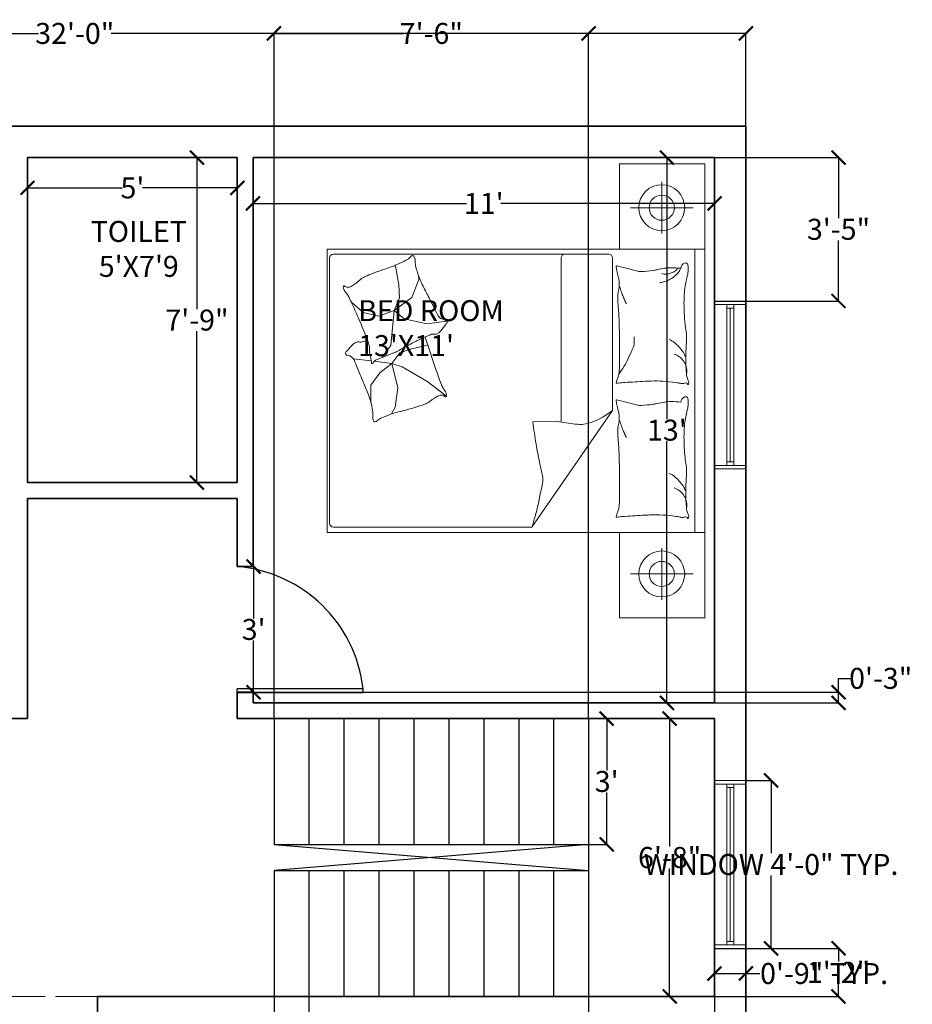
# Model space of a CAD drawing. Units: inches. Extents: x 43 to 543, y 36 to 629.
# Tile 5 of 5: x 261 to 516, y 348 to 629. Entities that reach past the tile are written whole.
import ezdxf

# ---------------------------------------------------------------- set-up
doc = ezdxf.new("R2010")
doc.units = ezdxf.units.IN
doc.header["$MEASUREMENT"] = 0
doc.linetypes.add('ACAD_ISO02W100', pattern=[15, 12, -3])
for name, color, linetype, lineweight in [('A-ANNO-DIMS', 2, 'Continuous', 18), ('A-AREA-IDEN', 7, 'Continuous', 25), ('A-DOOR', 3, 'Continuous', 25), ('A-FLOR-STRS', 7, 'Continuous', 25), ('A-FURN', 8, 'Continuous', 13), ('A-GLAZ', 4, 'Continuous', 18), ('A-WALL', 7, 'Continuous', 35), ('A-WALL-OVHD', 7, 'ACAD_ISO02W100', 18)]:
    doc.layers.add(name, color=color, linetype=linetype, lineweight=lineweight)
doc.styles.add('DIM_FONT', font='SIMPLEX.shx', dxfattribs={"width": 0.8})
doc.styles.get("Standard").update_dxf_attribs({"font": 'arial.ttf'})
doc.dimstyles.get("Standard").update_dxf_attribs({"dimtxt": 6, "dimasz": 4, "dimexe": 0.18, "dimexo": 0.0625, "dimgap": 0.09, "dimtad": 0, "dimtih": 1, "dimtoh": 1, "dimdec": 0, "dimzin": 0, "dimdsep": 46, "dimlunit": 4, "dimtxsty": 'Standard', "dimblk": 'ARCHTICK', "dimcen": 0.09, "dimadec": 0, "dimazin": 0, "dimtfac": 1, "dimtdec": 0, "dimtofl": 0, "dimtmove": 0, "dimatfit": 3, "dimldrblk": 'ARCHTICK', "dimfxl": 1, "dimtolj": 1, "dimtzin": 0, "dimarcsym": 1})

# ---------------------------------------------------------------- blocks, each defined once
blk = doc.blocks.new('XDCGFBHJNK')
for p, q in [((549.02, 46.3), (549.02, 41.8)), ((549.02, 46.3), (549.02, 10.3)), ((549.02, 46.3), (550.02, 46.3)), ((550.02, 10.3), (550.02, 46.3)), ((549.02, 10.3), (550.02, 10.3))]:
    blk.add_line(p, q)
blk.add_arc((545.53, 49.68), 39.64, 276.512, 355.1019)
blk = doc.blocks.new('TFHJBHN')
for p, q in [((347.02, 210.06), (338.02, 210.06)), ((347.02, 209.06), (338.02, 209.06)), ((341.52, 209.06), (341.52, 163.06)), ((343.52, 209.06), (343.52, 163.06)), ((343.52, 208.06), (341.52, 208.06)), ((342.52, 208.06), (342.52, 164.06)), ((341.52, 164.06), (343.52, 164.06)), ((338.02, 163.06), (347.02, 163.06)), ((338.02, 162.06), (347.02, 162.06))]:
    blk.add_line(p, q)
blk = doc.blocks.new('_ArchTick')
at = {"color": 0, "linetype": 'ByBlock', "const_width": 0.15}
blk.add_lwpolyline([(-0.5, -0.5), (0.5, 0.5)], dxfattribs=at)
blk = doc.blocks.new('*D4')
at = {"layer": 'A-ANNO-DIMS', "color": 0, "lineweight": -2, "transparency": 16777216}
for p, q in [((327.88, 589.95), (327.88, 576.71)), ((459.88, 589.95), (459.88, 576.71)), ((327.88, 576.89), (388.98, 576.89)), ((459.88, 576.89), (398.78, 576.89))]:
    blk.add_line(p, q, dxfattribs=at)
at = {"layer": 'Defpoints', "color": 0, "transparency": 16777216}
for p in [(327.88, 590.02), (459.88, 590.02), (459.88, 576.89)]:
    blk.add_point(p, dxfattribs=at)
at = {"layer": 'A-ANNO-DIMS', "color": 0, "lineweight": -2, "transparency": 16777216, "xscale": 4, "yscale": 4, "zscale": 4, "rotation": 180}
blk.add_blockref('_ArchTick', (327.88, 576.89), dxfattribs=at)
at = {"layer": 'A-ANNO-DIMS', "color": 0, "lineweight": -2, "transparency": 16777216, "xscale": 4, "yscale": 4, "zscale": 4}
blk.add_blockref('_ArchTick', (459.88, 576.89), dxfattribs=at)
at = {"layer": 'A-ANNO-DIMS', "color": 0, "transparency": 16777216, "insert": (393.88, 576.89), "char_height": 6, "attachment_point": 5}
blk.add_mtext("\\A1;11'", dxfattribs=at)
blk = doc.blocks.new('*D5')
at = {"layer": 'A-ANNO-DIMS', "color": 0, "lineweight": -2, "transparency": 16777216}
for p, q in [((459.82, 590.02), (446.09, 590.02)), ((446.27, 590.02), (446.27, 515.17)), ((446.27, 434.02), (446.27, 508.86)), ((459.82, 434.02), (446.09, 434.02))]:
    blk.add_line(p, q, dxfattribs=at)
at = {"layer": 'Defpoints', "color": 0, "transparency": 16777216}
for p in [(459.88, 590.02), (446.27, 434.02), (459.88, 434.02)]:
    blk.add_point(p, dxfattribs=at)
at = {"layer": 'A-ANNO-DIMS', "color": 0, "lineweight": -2, "transparency": 16777216, "xscale": 4, "yscale": 4, "zscale": 4}
for p, rotation in [((446.27, 590.02), 90), ((446.27, 434.02), 270)]:
    blk.add_blockref('_ArchTick', p, dxfattribs=dict(at, rotation=rotation))
at = {"layer": 'A-ANNO-DIMS', "color": 0, "transparency": 16777216, "insert": (446.27, 512.02), "char_height": 6, "attachment_point": 5}
blk.add_mtext("\\A1;13'", dxfattribs=at)
blk = doc.blocks.new('*D6')
at = {"layer": 'A-ANNO-DIMS', "color": 0, "lineweight": -2, "transparency": 16777216}
for p, q in [((263.38, 589.95), (263.38, 581.15)), ((323.38, 589.95), (323.38, 581.15)), ((263.38, 581.33), (290.53, 581.33)), ((323.38, 581.33), (296.23, 581.33))]:
    blk.add_line(p, q, dxfattribs=at)
at = {"layer": 'Defpoints', "color": 0, "transparency": 16777216}
for p in [(263.38, 590.02), (323.38, 590.02), (323.38, 581.33)]:
    blk.add_point(p, dxfattribs=at)
at = {"layer": 'A-ANNO-DIMS', "color": 0, "lineweight": -2, "transparency": 16777216, "xscale": 4, "yscale": 4, "zscale": 4, "rotation": 180}
blk.add_blockref('_ArchTick', (263.38, 581.33), dxfattribs=at)
at = {"layer": 'A-ANNO-DIMS', "color": 0, "lineweight": -2, "transparency": 16777216, "xscale": 4, "yscale": 4, "zscale": 4}
blk.add_blockref('_ArchTick', (323.38, 581.33), dxfattribs=at)
at = {"layer": 'A-ANNO-DIMS', "color": 0, "transparency": 16777216, "insert": (293.38, 581.33), "char_height": 6, "attachment_point": 5}
blk.add_mtext("\\A1;5'", dxfattribs=at)
blk = doc.blocks.new('*D7')
at = {"layer": 'A-ANNO-DIMS', "color": 0, "lineweight": -2, "transparency": 16777216}
for p, q in [((323.32, 590.02), (311.66, 590.02)), ((311.84, 590.02), (311.84, 546.67)), ((311.84, 497.02), (311.84, 540.36)), ((323.32, 497.02), (311.66, 497.02))]:
    blk.add_line(p, q, dxfattribs=at)
at = {"layer": 'Defpoints', "color": 0, "transparency": 16777216}
for p in [(323.38, 590.02), (311.84, 497.02), (323.38, 497.02)]:
    blk.add_point(p, dxfattribs=at)
at = {"layer": 'A-ANNO-DIMS', "color": 0, "lineweight": -2, "transparency": 16777216, "xscale": 4, "yscale": 4, "zscale": 4}
for p, rotation in [((311.84, 590.02), 90), ((311.84, 497.02), 270)]:
    blk.add_blockref('_ArchTick', p, dxfattribs=dict(at, rotation=rotation))
at = {"layer": 'A-ANNO-DIMS', "color": 0, "transparency": 16777216, "insert": (311.84, 543.52), "char_height": 6, "attachment_point": 5}
blk.add_mtext('\\A1;7\'-9"', dxfattribs=at)
blk = doc.blocks.new('*D16')
at = {"layer": 'A-ANNO-DIMS', "color": 0, "lineweight": -2, "transparency": 16777216}
for p, q in [((459.82, 429.52), (446.88, 429.52)), ((447.06, 429.52), (447.06, 392.92)), ((447.06, 350.02), (447.06, 386.61)), ((459.82, 350.02), (446.88, 350.02))]:
    blk.add_line(p, q, dxfattribs=at)
at = {"layer": 'Defpoints', "color": 0, "transparency": 16777216}
for p in [(459.88, 429.52), (447.06, 350.02), (459.88, 350.02)]:
    blk.add_point(p, dxfattribs=at)
at = {"layer": 'A-ANNO-DIMS', "color": 0, "lineweight": -2, "transparency": 16777216, "xscale": 4, "yscale": 4, "zscale": 4}
for p, rotation in [((447.06, 429.52), 90), ((447.06, 350.02), 270)]:
    blk.add_blockref('_ArchTick', p, dxfattribs=dict(at, rotation=rotation))
at = {"layer": 'A-ANNO-DIMS', "color": 0, "transparency": 16777216, "insert": (447.06, 389.77), "char_height": 6, "attachment_point": 5}
blk.add_mtext('\\A1;6\'-8"', dxfattribs=at)
blk = doc.blocks.new('*D17')
at = {"layer": 'A-ANNO-DIMS', "color": 0, "lineweight": -2, "transparency": 16777216}
for p, q in [((413.94, 429.52), (429.23, 429.52)), ((429.05, 429.52), (429.05, 414.67)), ((429.05, 393.52), (429.05, 408.36)), ((413.94, 393.52), (429.23, 393.52))]:
    blk.add_line(p, q, dxfattribs=at)
at = {"layer": 'Defpoints', "color": 0, "transparency": 16777216}
for p in [(413.88, 429.52), (413.88, 393.52), (429.05, 393.52)]:
    blk.add_point(p, dxfattribs=at)
at = {"layer": 'A-ANNO-DIMS', "color": 0, "lineweight": -2, "transparency": 16777216, "xscale": 4, "yscale": 4, "zscale": 4}
for p, rotation in [((429.05, 429.52), 90), ((429.05, 393.52), 270)]:
    blk.add_blockref('_ArchTick', p, dxfattribs=dict(at, rotation=rotation))
at = {"layer": 'A-ANNO-DIMS', "color": 0, "transparency": 16777216, "insert": (429.05, 411.52), "char_height": 6, "attachment_point": 5}
blk.add_mtext("\\A1;3'", dxfattribs=at)
blk = doc.blocks.new('*D18')
at = {"layer": 'A-ANNO-DIMS', "color": 0, "lineweight": -2, "transparency": 16777216}
for p, q in [((323.44, 473.02), (328.23, 473.02)), ((328.05, 473.02), (328.05, 458.17)), ((328.05, 437.02), (328.05, 451.86)), ((323.44, 437.02), (328.23, 437.02))]:
    blk.add_line(p, q, dxfattribs=at)
at = {"layer": 'Defpoints', "color": 0, "transparency": 16777216}
for p in [(323.38, 473.02), (323.38, 437.02), (328.05, 437.02)]:
    blk.add_point(p, dxfattribs=at)
at = {"layer": 'A-ANNO-DIMS', "color": 0, "lineweight": -2, "transparency": 16777216, "xscale": 4, "yscale": 4, "zscale": 4}
for p, rotation in [((328.05, 473.02), 90), ((328.05, 437.02), 270)]:
    blk.add_blockref('_ArchTick', p, dxfattribs=dict(at, rotation=rotation))
at = {"layer": 'A-ANNO-DIMS', "color": 0, "transparency": 16777216, "insert": (328.05, 455.02), "char_height": 6, "attachment_point": 5}
blk.add_mtext("\\A1;3'", dxfattribs=at)
blk = doc.blocks.new('BED-DOUBLE-WITH-NIGHTSTANDS')
for p, q in [((83.62, 105.4), (83.62, 129.79)), ((83.62, 129.79), (108, 129.79)), ((108, 129.79), (108, 105.4)), ((95.68, 109.93), (95.68, 124.65)), ((104.67, 117.29), (86.69, 117.29)), ((105.17, 105.4), (105.17, 24.4)), ((0.66, 102.92), (0.66, 27.01)), ((80.54, 104), (1.74, 104)), ((66.9, 102.92), (66.9, 55.97)), ((81.62, 59.31), (81.62, 102.92)), ((19.54, 100.52), (19.19, 100.7)), ((20.47, 95.22), (19.54, 100.52)), ((24.18, 91.6), (26.22, 96.71)), ((26.22, 96.71), (26.04, 98.01)), ((20.65, 91.51), (20.47, 95.22)), ((10.26, 87.33), (6.88, 90.22)), ((19.17, 87.89), (24.18, 91.6)), ((19.17, 87.89), (20.65, 91.51)), ((14.71, 86.21), (10.26, 87.33)), ((19.17, 87.89), (14.71, 86.21)), ((19.17, 87.89), (18.15, 77.85)), ((21.95, 85.47), (19.17, 87.89)), ((28.54, 84.08), (21.95, 85.47)), ((34.11, 84.82), (28.54, 84.08)), ((18.15, 77.85), (16.2, 75.16)), ((20.71, 75.8), (23.8, 76.86)), ((23.8, 76.86), (28.6, 77.93)), ((12.59, 73.43), (7.48, 74.07)), ((18.47, 72.7), (13.38, 73.34)), ((16.2, 75.16), (15.73, 74.51)), ((18.47, 72.7), (20.71, 75.8)), ((18.47, 72.7), (15.05, 70.03)), ((21.45, 71.74), (18.47, 72.7)), ((18.47, 72.7), (20.17, 65.76)), ((28.49, 67.68), (21.45, 71.74)), ((15.05, 70.03), (12.49, 66.51)), ((34.11, 63.41), (28.49, 67.68)), ((12.49, 66.51), (12.49, 61.49)), ((20.17, 65.76), (19.43, 60.21)), ((19.43, 60.21), (18.34, 58.27)), ((81.62, 59.31), (58.54, 25.93)), ((1.74, 25.93), (58.54, 25.93)), ((83.62, 24.4), (83.62, 0)), ((108, 0), (108, 24.4)), ((95.68, 19.86), (95.68, 5.14)), ((104.67, 12.5), (86.69, 12.5)), ((83.62, 0), (108, 0))]:
    blk.add_line(p, q)
blk.add_lwpolyline([(0, 105.4), (108, 105.4), (108, 24.4), (0, 24.4)], close=True)
blk.add_lwpolyline([(22.51, 102.26, 0.101392), (23.8, 103.26, -0.223768), (24.5, 103.58, -0.25558), (24.77, 103.43, -0.081563), (25.1, 102.61, -0.071805), (25.18, 101.69, 0.069985), (25.26, 100.74, 0.03546), (26.2, 97.59, 0.029432), (27.82, 93.98, 0.001554), (28.73, 92.24, -0.00152), (29.66, 90.47, -0.004735), (30.6, 88.63, 0.00382), (31.75, 86.35, 0.296001), (33.58, 85.3, -0.649774), (34.16, 84.19, -0.02319), (33.93, 83.92, 0.0288), (33.74, 83.71, 0.005727), (33.46, 83.33, -0.004358), (33.09, 82.83, -0.027528), (32.25, 81.85, -0.046214), (31.67, 81.34, -0.194121), (30.78, 81.12, 0.133719), (29.49, 80.96, 0.011505), (27.21, 79.95, 0.008882), (24.3, 78.53, 0.012426), (20.61, 76.53, -0.033612), (19.21, 75.84), (16.17, 74.6), (13.82, 73.64, 0.224341), (13.11, 72.86, -0.722772), (12.63, 72.85, -0.103513), (12.6, 73.05, 0.053465), (12.59, 73.44, 0.030109), (12.34, 74.68, -0.031436), (12.1, 75.88, -0.05324), (12.08, 76.69, 0.05518), (12.05, 77.48, 0.056271), (11.7, 78.85, 0.0108), (8.92, 85.64, 0.00456), (6.88, 90.22, 0.01125), (5.99, 92.05, 0.069394), (5.31, 93.02, -0.079756), (4.74, 93.88, -0.106399), (4.57, 94.66, -0.328642), (4.73, 94.89, -0.299547), (5.09, 94.79, 0.189917), (5.59, 94.53, 0.033518), (6.15, 94.51, 0.075627), (6.39, 94.55, 0.053489), (6.8, 94.74, 0.017838), (7.94, 95.49, 0.038394), (9.17, 96.51, -0.059529), (10, 97.14, -0.035943), (11.36, 97.82, -0.011245), (15.91, 99.56, -0.006203), (17.99, 100.27, 0.010783), (19.19, 100.7, 0.019485), (19.89, 100.99, 0.005062)], format="xyb", close=True)
for points in [[(101.15, 99.94, -0.263368), (102.17, 101.45, -0.494818), (103.18, 100.96, -0.049225), (103.27, 100, -0.036831), (103.18, 98.73, -0.031893), (102.74, 96.68, 0.035782), (102.36, 94.84, 0.032941), (102.04, 90, 0.026564), (102.36, 84, 0.017905), (102.65, 81.97, -0.033397), (102.77, 80.88, -0.03204), (102.73, 78.88, 0.018442), (102.57, 75.4, 0.010837), (102.61, 71.91, 0.014624), (102.77, 69.32, 0.111249), (103.17, 68.1, -0.153708), (103.38, 67.19, -0.076444), (103.29, 66.79, -0.215512), (103.18, 66.68, -0.585858), (103.02, 66.83, 0.363489), (102.88, 67.09, 0.191716), (102.25, 67.09, -0.129675), (101.36, 66.99, -0.01735), (100.45, 67.15, 0.019326), (99.63, 67.29, 0.018818), (95.94, 67.65, 0.021828), (92.74, 67.7, 0.006204), (90.91, 67.62, 0.001963), (85.14, 67.29, 0.028341), (83.19, 67.06, -0.117014), (82.71, 67.09, -0.36606), (82.66, 67.17, -0.03973), (82.81, 67.9, -0.048309), (83.11, 68.64, 0.062981), (83.32, 69.22, 0.04058), (83.5, 70.48, 0.014345), (83.62, 74.08, 0.005484), (83.58, 80.86, 0.007153), (83.42, 86.05, 0.008762), (83.27, 88.35, -0.008153), (83.12, 90.82, -0.06251), (83.35, 93.9, 0.078669), (83.46, 96.36, 0.047825), (83.21, 97.57, -0.034494), (82.81, 99.23, -0.023571), (82.65, 100.6, -0.510228), (82.71, 100.65), (84.33, 100.25), (88.79, 99.13, 0.073041), (89.85, 99.03, 0.023305), (93.15, 99.33, 0.018299), (94.38, 99.55, -0.01097), (96.43, 99.95, -0.042281), (98.29, 100.11, -0.027201), (101.17, 99.95)], [(101.15, 99.95, -0.077379), (99.79, 98.07, -0.077379), (97.91, 96.7, -0.047525), (96.58, 96.16, -0.047525), (95.17, 95.89)], [(100.29, 100.03, -0.05369), (99.59, 99.27, -0.070312), (98.92, 98.83, -0.015448), (98.46, 98.63, -0.013244), (97.91, 98.42, -0.082127), (96.93, 98.26, -0.064164), (95.68, 98.42)], [(83.5, 95.06, 0.009729), (83.99, 93.59, 0.009729), (84.53, 92.13, 0.007971), (85.02, 90.96, 0.007971), (85.55, 89.8)], [(28.06, 80.34, 0.025626), (28.21, 79.72, 0.0108), (30.46, 72.73, 0.00456), (32.14, 68.01, 0.01125), (32.88, 66.11, 0.069394), (33.49, 65.1, -0.079756), (33.99, 64.2, -0.106399), (34.11, 63.41, -0.328642), (33.92, 63.19, -0.299547), (33.57, 63.32, 0.189917), (33.1, 63.62, 0.033518), (32.54, 63.68, 0.075627), (32.29, 63.65, 0.053489), (31.87, 63.49, 0.017838), (30.68, 62.84, 0.038394), (29.37, 61.91, -0.059529), (28.5, 61.35, -0.035943), (27.09, 60.78, -0.011245), (22.42, 59.39, -0.006203), (20.29, 58.84, 0.010783), (19.06, 58.51, 0.019485), (18.34, 58.27, 0.005062), (15.63, 57.21, 0.101392), (14.27, 56.3, -0.223768), (13.54, 56.04, -0.25558), (13.29, 56.21, -0.081563), (13.02, 57.06, -0.071805), (13.01, 57.98, 0.069985), (13.01, 58.93, 0.03546), (12.31, 62.14, 0.029432), (10.97, 65.87, 0.001554), (10.2, 67.67, -0.00152), (9.41, 69.51, -0.004735), (8.61, 71.41, 0.00382), (7.64, 73.78, 0.296001), (5.89, 74.96, -0.649774), (5.41, 76.12, -0.02319), (5.66, 76.36, 0.0288), (5.85, 76.56, 0.005727), (6.17, 76.91, -0.004358), (6.58, 77.38, -0.027528), (7.49, 78.3, -0.046214), (8.1, 78.76, -0.194121), (9, 78.91, 0.133719), (10.3, 78.98, 0.005779), (11.49, 79.38, 0.008882)], [(83.42, 69.72, 0.016108), (84.84, 71.83, 0.024599), (85.65, 73.27, 0.009477), (86.91, 75.92, 0.015937), (87.57, 77.53, 0.072521), (87.77, 78.41, 0.033339), (87.78, 80.37)], [(102.57, 74.35, 0.027842), (101.99, 75.64, 0.048685), (101.56, 76.32, 0.023666), (100.24, 77.82, 0.031223), (99.13, 78.85, 0.046801), (98.71, 79.13, 0.023191), (97.81, 79.56)], [(102.88, 69.93, 0.088153), (102.68, 71.79, 0.088153), (101.86, 73.48, 0.077547), (100.7, 74.65, 0.077547), (99.23, 75.4)], [(101.15, 61.64, -0.263368), (102.17, 63.15, -0.494818), (103.18, 62.66, -0.049225), (103.27, 61.7, -0.036831), (103.18, 60.43, -0.031893), (102.74, 58.38, 0.035782), (102.36, 56.55, 0.032941), (102.04, 51.7, 0.026564), (102.36, 45.7, 0.017905), (102.65, 43.67, -0.033397), (102.77, 42.58, -0.03204), (102.73, 40.58, 0.018442), (102.57, 37.1, 0.010837), (102.61, 33.61, 0.014624), (102.77, 31.02, 0.111249), (103.17, 29.8, -0.153708), (103.38, 28.89, -0.076444), (103.29, 28.49, -0.215512), (103.18, 28.38, -0.585858), (103.02, 28.53, 0.363489), (102.88, 28.79, 0.191716), (102.25, 28.79, -0.129675), (101.36, 28.69, -0.01735), (100.45, 28.85, 0.019326), (99.63, 28.99, 0.018818), (95.94, 29.35, 0.021828), (92.74, 29.4, 0.006204), (90.91, 29.32, 0.001963), (85.14, 28.99, 0.028341), (83.19, 28.76, -0.117014), (82.71, 28.79, -0.36606), (82.66, 28.87, -0.03973), (82.81, 29.6, -0.048309), (83.11, 30.34, 0.062981), (83.32, 30.92, 0.04058), (83.5, 32.18, 0.014345), (83.62, 35.79, 0.005484), (83.58, 42.56, 0.007153), (83.42, 47.75, 0.008762), (83.27, 50.05, -0.008153), (83.12, 52.52, -0.06251), (83.35, 55.6, 0.078669), (83.46, 58.06, 0.047825), (83.21, 59.27, -0.034494), (82.81, 60.93, -0.023571), (82.65, 62.3, -0.510228), (82.71, 62.35), (84.33, 61.95), (88.79, 60.83, 0.073041), (89.85, 60.73, 0.023305), (93.15, 61.04, 0.018299), (94.38, 61.26, -0.01097), (96.43, 61.65, -0.042281), (98.29, 61.81, -0.027201), (101.17, 61.65)], [(81.62, 59.31, -0.085272), (75.67, 55.89, -0.124044), (70.95, 55.39), (65.79, 56.13), (58.77, 56.03)], [(83.5, 56.76, 0.009729), (83.99, 55.29, 0.009729), (84.53, 53.84, 0.007971), (85.02, 52.66, 0.007971), (85.55, 51.5)], [(58.77, 56.03, 0.007867), (59.73, 49.68, 0.009508), (60.7, 44.46, 0.006616), (61.48, 40.95, -0.023828), (61.66, 39.97, -0.080713), (61.63, 38.96, -0.009591), (59.91, 30.72, -0.013133), (59.44, 28.91, -0.007859), (58.54, 25.93)], [(102.57, 36.06, 0.027842), (101.99, 37.34, 0.048685), (101.56, 38.02, 0.023666), (100.24, 39.52, 0.031223), (99.13, 40.55, 0.046801), (98.71, 40.83, 0.023191), (97.81, 41.26)], [(102.88, 31.63, 0.088153), (102.68, 33.49, 0.088153), (101.86, 35.18, 0.077547), (100.7, 36.35, 0.077547), (99.23, 37.1)]]:
    blk.add_lwpolyline(points, format="xyb")
for centre, radius in [((95.68, 117.29), 6.58), ((95.68, 117.29), 3.6), ((95.68, 12.5), 6.58), ((95.68, 12.5), 3.6)]:
    blk.add_circle(centre, radius)
for centre, start, end in [((1.74, 102.92), 90, 180), ((67.98, 102.92), 90, 180), ((80.54, 102.92), 0, 90), ((1.74, 27.01), 180, 270)]:
    blk.add_arc(centre, 1.08, start, end)
at = {"style": 'DIM_FONT', "width": 0.8, "flags": 9}
for tag in ['YSIZE', 'XSIZE']:
    blk.add_attdef(tag, (108, 105.4), '', height=0.027, rotation=270, dxfattribs=at)
blk = doc.blocks.new('*D35')
at = {"layer": 'A-ANNO-DIMS', "color": 0, "lineweight": -2, "transparency": 16777216}
for p, q in [((468.94, 411.78), (476.26, 411.78)), ((476.08, 411.78), (476.08, 390.98)), ((476.08, 363.78), (476.08, 384.59)), ((468.94, 363.78), (476.26, 363.78))]:
    blk.add_line(p, q, dxfattribs=at)
at = {"layer": 'Defpoints', "color": 0, "transparency": 16777216}
for p in [(468.88, 411.78), (476.08, 411.78), (468.88, 363.78)]:
    blk.add_point(p, dxfattribs=at)
at = {"layer": 'A-ANNO-DIMS', "color": 0, "lineweight": -2, "transparency": 16777216, "xscale": 4, "yscale": 4, "zscale": 4}
for p, rotation in [((476.08, 411.78), 90), ((476.08, 363.78), 270)]:
    blk.add_blockref('_ArchTick', p, dxfattribs=dict(at, rotation=rotation))
at = {"layer": 'A-ANNO-DIMS', "color": 0, "transparency": 16777216, "insert": (476.08, 387.78), "char_height": 6, "attachment_point": 5}
blk.add_mtext('\\A1;WINDOW 4\'-0" TYP.', dxfattribs=at)
blk = doc.blocks.new('*D36')
at = {"layer": 'A-ANNO-DIMS', "color": 0, "lineweight": -2, "transparency": 16777216}
for p, q in [((459.88, 363.72), (459.88, 356.4)), ((468.88, 363.72), (468.88, 356.4)), ((459.88, 356.58), (468.88, 356.58)), ((468.88, 356.58), (472.88, 356.58))]:
    blk.add_line(p, q, dxfattribs=at)
at = {"layer": 'Defpoints', "color": 0, "transparency": 16777216}
for p in [(459.88, 363.78), (468.88, 363.78), (468.88, 356.58)]:
    blk.add_point(p, dxfattribs=at)
at = {"layer": 'A-ANNO-DIMS', "color": 0, "lineweight": -2, "transparency": 16777216, "xscale": 4, "yscale": 4, "zscale": 4, "rotation": 180}
blk.add_blockref('_ArchTick', (459.88, 356.58), dxfattribs=at)
at = {"layer": 'A-ANNO-DIMS', "color": 0, "lineweight": -2, "transparency": 16777216, "xscale": 4, "yscale": 4, "zscale": 4}
blk.add_blockref('_ArchTick', (468.88, 356.58), dxfattribs=at)
at = {"layer": 'A-ANNO-DIMS', "color": 0, "transparency": 16777216, "insert": (491.25, 356.58), "char_height": 6, "attachment_point": 5}
blk.add_mtext('\\A1;0\'-9" TYP.', dxfattribs=at)
blk = doc.blocks.new('*D37')
at = {"layer": 'A-ANNO-DIMS', "color": 0, "lineweight": -2, "transparency": 16777216}
for p, q in [((84.88, 599.08), (84.88, 625.7)), ((84.88, 625.52), (266.48, 625.52)), ((468.88, 625.52), (287.27, 625.52)), ((468.88, 599.08), (468.88, 625.7))]:
    blk.add_line(p, q, dxfattribs=at)
at = {"layer": 'Defpoints', "color": 0, "transparency": 16777216}
for p in [(468.88, 625.52), (84.88, 599.02), (468.88, 599.02)]:
    blk.add_point(p, dxfattribs=at)
at = {"layer": 'A-ANNO-DIMS', "color": 0, "lineweight": -2, "transparency": 16777216, "xscale": 4, "yscale": 4, "zscale": 4, "rotation": 180}
blk.add_blockref('_ArchTick', (84.88, 625.52), dxfattribs=at)
at = {"layer": 'A-ANNO-DIMS', "color": 0, "lineweight": -2, "transparency": 16777216, "xscale": 4, "yscale": 4, "zscale": 4}
blk.add_blockref('_ArchTick', (468.88, 625.52), dxfattribs=at)
at = {"layer": 'A-ANNO-DIMS', "color": 0, "transparency": 16777216, "insert": (276.88, 625.52), "char_height": 6, "attachment_point": 5}
blk.add_mtext('\\A1;32\'-0"', dxfattribs=at)
blk = doc.blocks.new('*D39')
at = {"layer": 'A-ANNO-DIMS', "color": 0, "lineweight": -2, "transparency": 16777216}
for p, q in [((459.94, 590.02), (495.56, 590.02)), ((495.38, 590.02), (495.38, 572.64)), ((495.38, 548.96), (495.38, 566.33)), ((459.94, 548.96), (495.56, 548.96))]:
    blk.add_line(p, q, dxfattribs=at)
at = {"layer": 'Defpoints', "color": 0, "transparency": 16777216}
for p in [(459.88, 590.02), (459.88, 548.96), (495.38, 548.96)]:
    blk.add_point(p, dxfattribs=at)
at = {"layer": 'A-ANNO-DIMS', "color": 0, "lineweight": -2, "transparency": 16777216, "xscale": 4, "yscale": 4, "zscale": 4}
for p, rotation in [((495.38, 590.02), 90), ((495.38, 548.96), 270)]:
    blk.add_blockref('_ArchTick', p, dxfattribs=dict(at, rotation=rotation))
at = {"layer": 'A-ANNO-DIMS', "color": 0, "transparency": 16777216, "insert": (495.38, 569.49), "char_height": 6, "attachment_point": 5}
blk.add_mtext('\\A1;3\'-5"', dxfattribs=at)
blk = doc.blocks.new('*D40')
at = {"layer": 'A-ANNO-DIMS', "color": 0, "lineweight": -2, "transparency": 16777216}
for p, q in [((459.94, 363.78), (495.56, 363.78)), ((495.38, 363.78), (495.38, 360)), ((495.38, 350.02), (495.38, 353.8)), ((459.94, 350.02), (495.56, 350.02))]:
    blk.add_line(p, q, dxfattribs=at)
at = {"layer": 'Defpoints', "color": 0, "transparency": 16777216}
for p in [(459.88, 363.78), (495.38, 363.78), (459.88, 350.02)]:
    blk.add_point(p, dxfattribs=at)
at = {"layer": 'A-ANNO-DIMS', "color": 0, "lineweight": -2, "transparency": 16777216, "xscale": 4, "yscale": 4, "zscale": 4}
for p, rotation in [((495.38, 363.78), 90), ((495.38, 350.02), 270)]:
    blk.add_blockref('_ArchTick', p, dxfattribs=dict(at, rotation=rotation))
at = {"layer": 'A-ANNO-DIMS', "color": 0, "transparency": 16777216, "insert": (495.38, 356.9), "char_height": 6, "attachment_point": 5}
blk.add_mtext('\\A1;1\'-2"', dxfattribs=at)
blk = doc.blocks.new('*D46')
at = {"layer": 'A-ANNO-DIMS', "color": 0, "lineweight": -2, "transparency": 16777216}
for p, q in [((333.88, 429.58), (333.88, 625.7)), ((333.88, 625.52), (370.84, 625.52)), ((423.88, 625.52), (386.92, 625.52)), ((423.88, 429.58), (423.88, 625.7))]:
    blk.add_line(p, q, dxfattribs=at)
at = {"layer": 'Defpoints', "color": 0, "transparency": 16777216}
for p in [(423.88, 625.52), (333.88, 429.52), (423.88, 429.52)]:
    blk.add_point(p, dxfattribs=at)
at = {"layer": 'A-ANNO-DIMS', "color": 0, "lineweight": -2, "transparency": 16777216, "xscale": 4, "yscale": 4, "zscale": 4, "rotation": 180}
blk.add_blockref('_ArchTick', (333.88, 625.52), dxfattribs=at)
at = {"layer": 'A-ANNO-DIMS', "color": 0, "lineweight": -2, "transparency": 16777216, "xscale": 4, "yscale": 4, "zscale": 4}
blk.add_blockref('_ArchTick', (423.88, 625.52), dxfattribs=at)
at = {"layer": 'A-ANNO-DIMS', "color": 0, "transparency": 16777216, "insert": (378.88, 625.52), "char_height": 6, "attachment_point": 5}
blk.add_mtext('\\A1;7\'-6"', dxfattribs=at)
blk = doc.blocks.new('*D47')
at = {"layer": 'A-ANNO-DIMS', "color": 0, "lineweight": -2, "transparency": 16777216}
for p, q in [((423.88, 349.95), (423.88, 44.34)), ((459.88, 349.95), (459.88, 44.34)), ((423.88, 44.52), (433.81, 44.52)), ((459.88, 44.52), (449.94, 44.52))]:
    blk.add_line(p, q, dxfattribs=at)
at = {"layer": 'Defpoints', "color": 0, "transparency": 16777216}
for p in [(423.88, 350.02), (459.88, 350.02), (459.88, 44.52)]:
    blk.add_point(p, dxfattribs=at)
at = {"layer": 'A-ANNO-DIMS', "color": 0, "lineweight": -2, "transparency": 16777216, "xscale": 4, "yscale": 4, "zscale": 4, "rotation": 180}
blk.add_blockref('_ArchTick', (423.88, 44.52), dxfattribs=at)
at = {"layer": 'A-ANNO-DIMS', "color": 0, "lineweight": -2, "transparency": 16777216, "xscale": 4, "yscale": 4, "zscale": 4}
blk.add_blockref('_ArchTick', (459.88, 44.52), dxfattribs=at)
at = {"layer": 'A-ANNO-DIMS', "color": 0, "transparency": 16777216, "insert": (441.88, 44.52), "char_height": 6, "attachment_point": 5}
blk.add_mtext('\\A1;3\'-0"', dxfattribs=at)
blk = doc.blocks.new('*D48')
at = {"layer": 'A-ANNO-DIMS', "color": 0, "lineweight": -2, "transparency": 16777216}
for p, q in [((333.88, 349.95), (333.88, 44.34)), ((343.88, 349.95), (343.88, 44.34)), ((333.88, 44.52), (343.88, 44.52)), ((343.88, 44.52), (347.88, 44.52))]:
    blk.add_line(p, q, dxfattribs=at)
at = {"layer": 'Defpoints', "color": 0, "transparency": 16777216}
for p in [(333.88, 350.02), (343.88, 350.02), (343.88, 44.52)]:
    blk.add_point(p, dxfattribs=at)
at = {"layer": 'A-ANNO-DIMS', "color": 0, "lineweight": -2, "transparency": 16777216, "xscale": 4, "yscale": 4, "zscale": 4, "rotation": 180}
blk.add_blockref('_ArchTick', (333.88, 44.52), dxfattribs=at)
at = {"layer": 'A-ANNO-DIMS', "color": 0, "lineweight": -2, "transparency": 16777216, "xscale": 4, "yscale": 4, "zscale": 4}
blk.add_blockref('_ArchTick', (343.88, 44.52), dxfattribs=at)
at = {"layer": 'A-ANNO-DIMS', "color": 0, "transparency": 16777216, "insert": (358.27, 44.52), "char_height": 6, "attachment_point": 5}
blk.add_mtext('\\A1;0\'-10"', dxfattribs=at)
blk = doc.blocks.new('*D63')
at = {"layer": 'A-ANNO-DIMS', "color": 0, "lineweight": -2, "transparency": 16777216}
for p, q in [((495.38, 437.02), (495.38, 441.02)), ((495.38, 441.02), (499.38, 441.02)), ((327.94, 437.02), (495.56, 437.02)), ((495.38, 434.02), (495.38, 437.02)), ((327.94, 434.02), (495.56, 434.02))]:
    blk.add_line(p, q, dxfattribs=at)
at = {"layer": 'Defpoints', "color": 0, "transparency": 16777216}
for p in [(327.88, 437.02), (495.38, 437.02), (327.88, 434.02)]:
    blk.add_point(p, dxfattribs=at)
at = {"layer": 'A-ANNO-DIMS', "color": 0, "lineweight": -2, "transparency": 16777216, "xscale": 4, "yscale": 4, "zscale": 4}
for p, rotation in [((495.38, 437.02), 90), ((495.38, 434.02), 270)]:
    blk.add_blockref('_ArchTick', p, dxfattribs=dict(at, rotation=rotation))
at = {"layer": 'A-ANNO-DIMS', "color": 0, "transparency": 16777216, "insert": (507.44, 441.02), "char_height": 6, "attachment_point": 5}
blk.add_mtext('\\A1;0\'-3"', dxfattribs=at)

msp = doc.modelspace()

# ---------------------------------------------------------------- linework, layer by layer
at = {"layer": 'A-FLOR-STRS'}
for p, q in [((333.88, 429.52), (333.88, 393.52)), ((343.88, 429.52), (343.88, 393.52)), ((353.88, 429.52), (353.88, 393.52)), ((363.88, 429.52), (363.88, 393.52)), ((373.88, 429.52), (373.88, 393.52)), ((383.88, 429.52), (383.88, 393.52)), ((393.88, 429.52), (393.88, 393.52)), ((403.88, 429.52), (403.88, 393.52)), ((413.88, 429.52), (413.88, 393.52)), ((423.88, 429.52), (423.88, 350.02)), ((333.88, 393.52), (423.88, 393.52)), ((423.88, 393.52), (333.88, 386.02)), ((333.88, 393.52), (423.88, 386.02)), ((333.88, 386.02), (423.88, 386.02)), ((333.88, 386.02), (333.88, 350.02)), ((343.88, 386.02), (343.88, 350.02)), ((353.88, 386.02), (353.88, 350.02)), ((363.88, 386.02), (363.88, 350.02)), ((373.88, 386.02), (373.88, 350.02)), ((383.88, 386.02), (383.88, 350.02)), ((393.88, 386.02), (393.88, 350.02)), ((403.88, 386.02), (403.88, 350.02)), ((413.88, 386.02), (413.88, 350.02))]:
    msp.add_line(p, q, dxfattribs=at)
at = {"layer": 'A-WALL'}
for p, q in [((84.88, 599.02), (468.88, 599.02)), ((468.88, 599.02), (468.88, 71.02)), ((263.38, 590.02), (263.38, 497.02)), ((263.38, 590.02), (323.38, 590.02)), ((323.38, 590.02), (323.38, 497.02)), ((327.88, 590.02), (327.88, 473.02)), ((327.88, 590.02), (459.88, 590.02)), ((459.88, 590.02), (459.88, 434.02)), ((323.38, 497.02), (263.38, 497.02)), ((323.38, 492.52), (263.38, 492.52)), ((263.38, 492.52), (263.38, 429.52)), ((323.38, 492.52), (323.38, 473.02)), ((323.38, 473.02), (327.88, 473.02)), ((323.38, 437.02), (327.88, 437.02)), ((323.38, 437.02), (323.38, 429.52)), ((327.88, 437.02), (327.88, 434.02)), ((327.88, 434.02), (459.88, 434.02)), ((258.88, 429.52), (263.38, 429.52)), ((323.38, 429.52), (459.88, 429.52)), ((459.88, 429.52), (459.88, 350.02)), ((283.38, 350.02), (283.38, 345.52)), ((283.38, 350.02), (459.88, 350.02))]:
    msp.add_line(p, q, dxfattribs=at)
at = {"layer": 'A-WALL-OVHD'}
msp.add_line((283.38, 350.02), (223.38, 350.02), dxfattribs=at)

# ---------------------------------------------------------------- block references
at = {"layer": 'A-DOOR', "rotation": 90}
msp.add_blockref('XDCGFBHJNK', (369.67, -112.01), dxfattribs=at)
at = {"layer": 'A-FURN'}
msp.add_blockref('BED-DOUBLE-WITH-NIGHTSTANDS', (349.13, 458.38), dxfattribs=at)
at = {"layer": 'A-GLAZ'}
for p in [(121.86, 338.9), (121.86, 201.72)]:
    msp.add_blockref('TFHJBHN', p, dxfattribs=at)

# ---------------------------------------------------------------- texts
at = {"layer": 'A-AREA-IDEN', "char_height": 6, "attachment_point": 1}
for s, width, insert in [("\\pxqc;TOILET\\P5'X7'9", 52.429, (268.98, 571.88)), ("BED ROOM\\P13'X11' ", 90.4757, (357.95, 549.21))]:
    msp.add_mtext_dynamic_manual_height_columns(s, width=width, gutter_width=30, heights=[0], dxfattribs=dict(at, insert=insert))

# ---------------------------------------------------------------- dimensions: what is measured, and where the dimension line sits
at = {"layer": 'A-ANNO-DIMS'}
for base, p1, p2, override, picture, middle in [((468.88, 625.52), (84.88, 599.02), (468.88, 599.02), {"dimdec": 1, "dimlfac": 1, "dimrnd": 0, "dimzin": 1, "dimdsep": 46, "dimlunit": 4, "dimfrac": 2}, '*D37', (276.88, 625.52)), ((423.88, 625.52), (333.88, 429.52), (423.88, 429.52), {"dimdec": 1, "dimlfac": 1, "dimrnd": 0, "dimzin": 1, "dimdsep": 46, "dimlunit": 4, "dimfrac": 2}, '*D46', (378.88, 625.52)), ((323.38, 581.33), (263.38, 590.02), (323.38, 590.02), {"dimclrd": 0, "dimclre": 0, "dimclrt": 0}, '*D6', (293.38, 581.33)), ((459.88, 576.89), (327.88, 590.02), (459.88, 590.02), {"dimclrd": 0, "dimclre": 0, "dimclrt": 0}, '*D4', (393.88, 576.89)), ((343.88, 44.52), (333.88, 350.02), (343.88, 350.02), {"dimdec": 1, "dimlfac": 1, "dimrnd": 0, "dimzin": 1, "dimdsep": 46, "dimlunit": 4, "dimfrac": 2}, '*D48', (358.27, 44.52)), ((459.88, 44.52), (423.88, 350.02), (459.88, 350.02), {"dimdec": 1, "dimlfac": 1, "dimrnd": 0, "dimzin": 1, "dimdsep": 46, "dimlunit": 4, "dimfrac": 2}, '*D47', (441.88, 44.52))]:
    dim = msp.add_linear_dim(base=base, p1=p1, p2=p2, dimstyle='Standard', override=override, dxfattribs=at)
    dim.commit()
    dim.dimension.update_dxf_attribs({"geometry": picture, "text_midpoint": middle})
for base, p1, p2, override, picture, middle in [((311.84, 497.02), (323.38, 590.02), (323.38, 497.02), {"dimclrd": 0, "dimclre": 0, "dimclrt": 0}, '*D7', (311.84, 543.52)), ((446.27, 434.02), (459.88, 590.02), (459.88, 434.02), {"dimclrd": 0, "dimclre": 0, "dimclrt": 0}, '*D5', (446.27, 512.02)), ((495.38, 548.96), (459.88, 590.02), (459.88, 548.96), {"dimdec": 1, "dimlfac": 1, "dimrnd": 0, "dimzin": 1, "dimdsep": 46, "dimlunit": 4, "dimfrac": 2}, '*D39', (495.38, 569.49)), ((328.05, 437.02), (323.38, 473.02), (323.38, 437.02), {"dimclrd": 0, "dimclre": 0, "dimclrt": 0}, '*D18', (328.05, 455.02)), ((495.38, 437.02), (327.88, 434.02), (327.88, 437.02), {"dimdec": 1, "dimlfac": 1, "dimrnd": 0, "dimzin": 1, "dimdsep": 46, "dimlunit": 4, "dimfrac": 2}, '*D63', (507.44, 441.02)), ((429.05, 393.52), (413.88, 429.52), (413.88, 393.52), {"dimclrd": 0, "dimclre": 0, "dimclrt": 0}, '*D17', (429.05, 411.52)), ((447.06164371, 350.01657912), (459.877649, 429.51657912), (459.877649, 350.01657912), {"dimclrd": 0, "dimclre": 0, "dimclrt": 0}, '*D16', (447.06164371, 389.76657912)), ((495.38, 363.78), (459.88, 350.02), (459.88, 363.78), {"dimdec": 1, "dimlfac": 1, "dimrnd": 0, "dimzin": 1, "dimdsep": 46, "dimlunit": 4, "dimfrac": 2}, '*D40', (495.38, 356.9))]:
    dim = msp.add_linear_dim(base=base, p1=p1, p2=p2, angle=90, dimstyle='Standard', override=override, dxfattribs=at)
    dim.commit()
    dim.dimension.update_dxf_attribs({"geometry": picture, "text_midpoint": middle})
dim = msp.add_linear_dim(base=(476.08, 411.78), p1=(468.88, 363.78), p2=(468.88, 411.78), angle=90, text='WINDOW <> TYP.', dimstyle='Standard', override={"dimdec": 1, "dimlfac": 1, "dimrnd": 0, "dimzin": 1, "dimdsep": 46, "dimlunit": 4, "dimfrac": 2}, dxfattribs=at)
dim.commit()
dim.dimension.update_dxf_attribs({"geometry": '*D35', "text_midpoint": (476.08, 387.78)})
dim = msp.add_linear_dim(base=(468.88, 356.58), p1=(459.88, 363.78), p2=(468.88, 363.78), text='<> TYP.', dimstyle='Standard', override={"dimdec": 1, "dimlfac": 1, "dimrnd": 0, "dimzin": 1, "dimdsep": 46, "dimlunit": 4, "dimfrac": 2}, dxfattribs=at)
dim.commit()
dim.dimension.update_dxf_attribs({"geometry": '*D36', "text_midpoint": (491.25, 356.58)})

doc.saveas('drawing.dxf')
